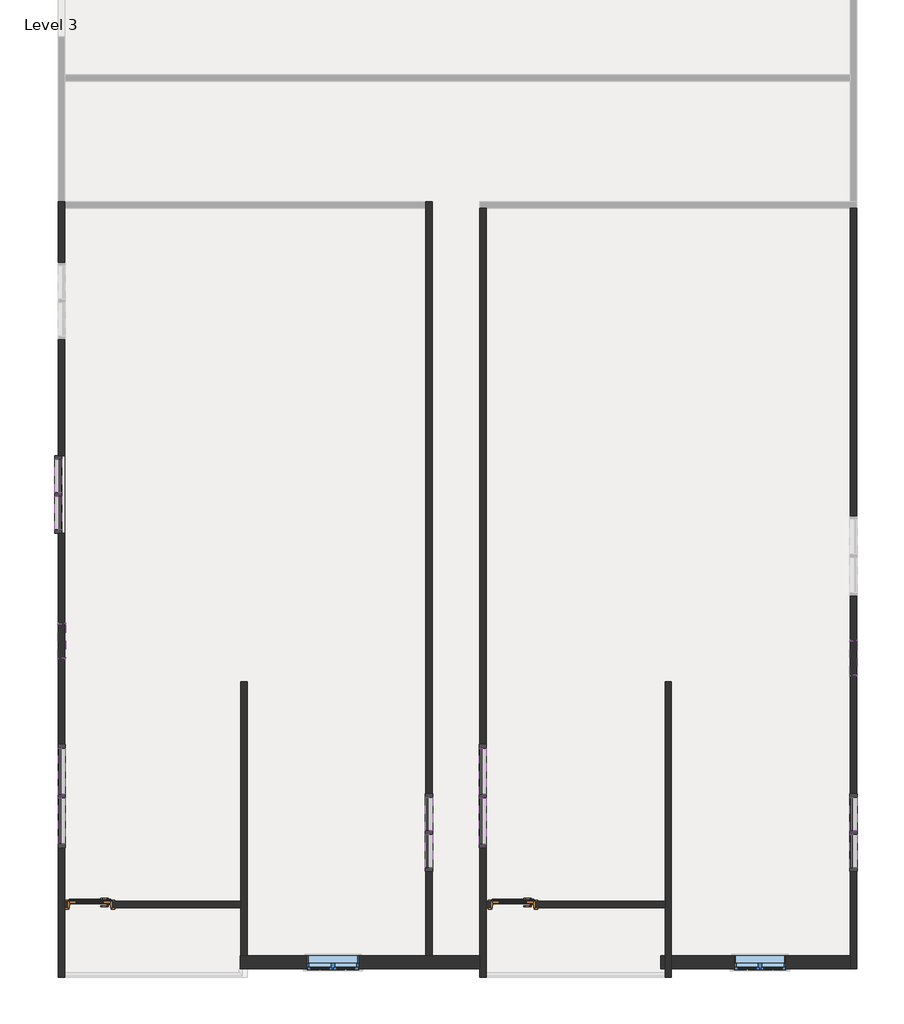
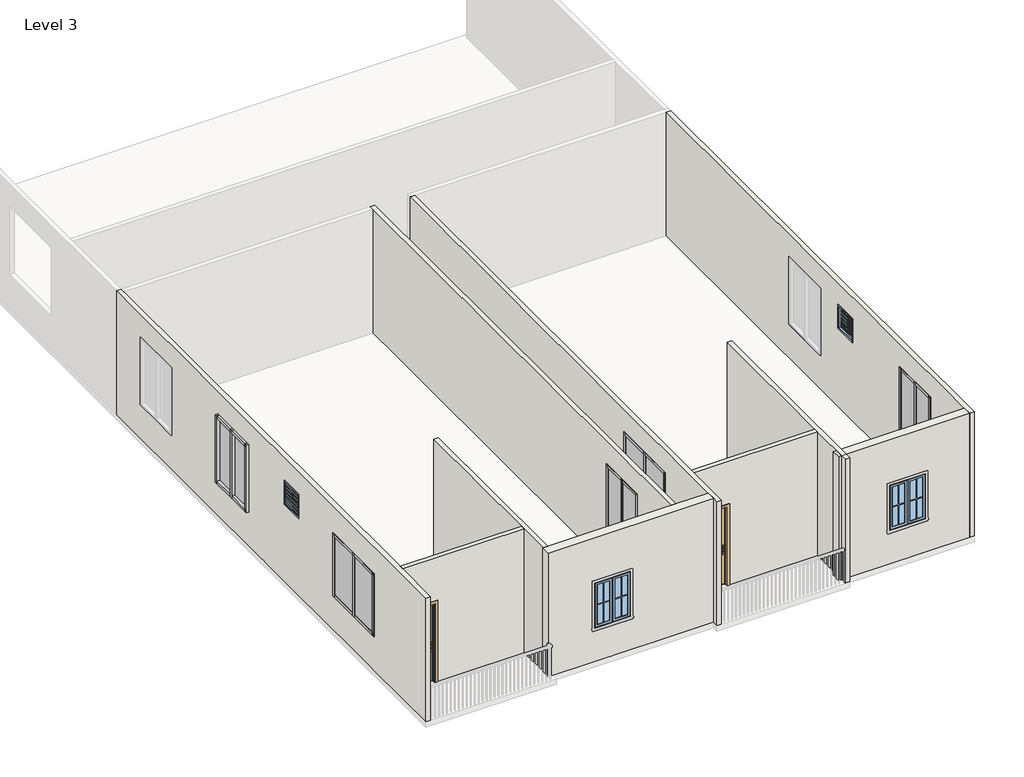
# One storey, part 1 of 3: 35 members, 10 plates, 10 walls, 4 windows, 2 doors.
"""IFC4 building model written with IfcOpenShell, lengths in millimetres."""

from ifc_helpers import new_model, si_unit, frame, origin, place, context, project, spatial, polyline, outline, extrude, faceted_brep, transform, mapped, element, save
from components import door_b81be692, member_8acf8d94, member_501b078b, member_2e6d4a6b, member_96ae0c19, member_d60e8053, member_2fae0574, member_b8ac15de, member_17644e48, system_panel_glazed_c4393626, system_panel_glazed_0e71bc1b, system_panel_glazed_e97abd02, system_panel_glazed_a7ecbca6, window_d341e8ac, window_d39e7ecb

model = new_model("IFC4")

# Units and contexts
model_context = context("Model", 3, world=origin())
ifc_project = project(units=[si_unit("LENGTHUNIT", "METRE", prefix="MILLI")], contexts=[model_context])

# Site, building, storey
site = spatial("IfcSite", under=ifc_project)
building = spatial("IfcBuilding", under=site)
storey = spatial("IfcBuildingStorey", under=building, Name="Level 3", Elevation=6705.6)

# Doors
placement = place(None, origin())
door_shape = door_b81be692(model_context)
element("IfcDoor", 1, ObjectType="29\" x 84\"", at=placement, inside=storey, context=model_context, shape_type="MappedRepresentation", body=[
    mapped(door_shape, transform((-7651.507583, -9448.7163489, 6705.6), x_axis=(1.0, 0.0, 0.0), y_axis=(0.0, 1.0, 0.0), z_axis=(0.0, 0.0, 1.0))),
])
element("IfcDoor", 2, ObjectType="29\" x 84\"", at=placement, inside=storey, context=model_context, shape_type="MappedRepresentation", body=[
    mapped(door_shape, transform((-172.2931282, -9448.9038009, 6705.6), x_axis=(1.0, 0.0, 0.0), y_axis=(0.0, 1.0, 0.0), z_axis=(0.0, 0.0, 1.0))),
])

# Members
member_shape = member_8acf8d94(model_context)
element("IfcMember", 3, ObjectType="Rectangular Mullion : 2.5\" x 5\" rectangular", at=placement, inside=storey, context=model_context, shape_type="MappedRepresentation", body=[
    mapped(member_shape, transform((-8153.157583, -8377.1401329, 9327.486558), x_axis=(0.0, 0.0, 1.0), y_axis=(-1.0, 0.0, 0.0), z_axis=(0.0, -1.0, 0.0))),
])
element("IfcMember", 4, ObjectType="Rectangular Mullion : 2.5\" x 5\" rectangular", at=placement, inside=storey, context=model_context, shape_type="MappedRepresentation", body=[
    mapped(member_shape, transform((-8153.157583, -7497.6651329, 9327.486558), x_axis=(0.0, 0.0, 1.0), y_axis=(-1.0, 0.0, 0.0), z_axis=(0.0, -1.0, 0.0))),
])
element("IfcMember", 5, ObjectType="Rectangular Mullion : 2.5\" x 5\" rectangular", at=placement, inside=storey, context=model_context, shape_type="MappedRepresentation", body=[
    mapped(member_shape, transform((-8153.157583, -6681.6901329, 7620.0), x_axis=(0.0, 0.0, -1.0), y_axis=(-1.0, 0.0, 0.0), z_axis=(0.0, 1.0, 0.0))),
])
element("IfcMember", 6, ObjectType="Rectangular Mullion : 2.5\" x 5\" rectangular", at=placement, inside=storey, context=model_context, shape_type="MappedRepresentation", body=[
    mapped(member_shape, transform((-8153.157583, -7561.1651329, 7620.0), x_axis=(0.0, 0.0, -1.0), y_axis=(-1.0, 0.0, 0.0), z_axis=(0.0, 1.0, 0.0))),
])
member_2_shape = member_501b078b(model_context)
element("IfcMember", 7, ObjectType="Rectangular Mullion : 2.5\" x 5\" rectangular", at=placement, inside=storey, context=model_context, shape_type="MappedRepresentation", body=[
    mapped(member_2_shape, transform((5848.1708786, -8795.0998253, 9448.8), x_axis=(0.0, 0.0, 1.0), y_axis=(-1.0, 0.0, 0.0), z_axis=(0.0, -1.0, 0.0))),
])
element("IfcMember", 8, ObjectType="Rectangular Mullion : 2.5\" x 5\" rectangular", at=placement, inside=storey, context=model_context, shape_type="MappedRepresentation", body=[
    mapped(member_2_shape, transform((5848.1708786, -8142.1745373, 9448.8), x_axis=(0.0, 0.0, 1.0), y_axis=(-1.0, 0.0, 0.0), z_axis=(0.0, -1.0, 0.0))),
])
element("IfcMember", 9, ObjectType="Rectangular Mullion : 2.5\" x 5\" rectangular", at=placement, inside=storey, context=model_context, shape_type="MappedRepresentation", body=[
    mapped(member_2_shape, transform((-1656.4435762, -8795.0998253, 9448.8), x_axis=(0.0, 0.0, 1.0), y_axis=(-1.0, 0.0, 0.0), z_axis=(0.0, -1.0, 0.0))),
])
element("IfcMember", 10, ObjectType="Rectangular Mullion : 2.5\" x 5\" rectangular", at=placement, inside=storey, context=model_context, shape_type="MappedRepresentation", body=[
    mapped(member_2_shape, transform((-1656.4435762, -8142.1745373, 9448.8), x_axis=(0.0, 0.0, 1.0), y_axis=(-1.0, 0.0, 0.0), z_axis=(0.0, -1.0, 0.0))),
])
element("IfcMember", 11, ObjectType="Rectangular Mullion : 2.5\" x 5\" rectangular", at=placement, inside=storey, context=model_context, shape_type="MappedRepresentation", body=[
    mapped(member_2_shape, transform((5848.1708786, -7552.7492493, 7620.0), x_axis=(0.0, 0.0, -1.0), y_axis=(-1.0, 0.0, 0.0), z_axis=(0.0, 1.0, 0.0))),
])
element("IfcMember", 12, ObjectType="Rectangular Mullion : 2.5\" x 5\" rectangular", at=placement, inside=storey, context=model_context, shape_type="MappedRepresentation", body=[
    mapped(member_2_shape, transform((5848.1708786, -8205.6745373, 7620.0), x_axis=(0.0, 0.0, -1.0), y_axis=(-1.0, 0.0, 0.0), z_axis=(0.0, 1.0, 0.0))),
])
element("IfcMember", 13, ObjectType="Rectangular Mullion : 2.5\" x 5\" rectangular", at=placement, inside=storey, context=model_context, shape_type="MappedRepresentation", body=[
    mapped(member_2_shape, transform((-1656.4435762, -7552.7492493, 7620.0), x_axis=(0.0, 0.0, -1.0), y_axis=(-1.0, 0.0, 0.0), z_axis=(0.0, 1.0, 0.0))),
])
element("IfcMember", 14, ObjectType="Rectangular Mullion : 2.5\" x 5\" rectangular", at=placement, inside=storey, context=model_context, shape_type="MappedRepresentation", body=[
    mapped(member_2_shape, transform((-1656.4435762, -8205.6745373, 7620.0), x_axis=(0.0, 0.0, -1.0), y_axis=(-1.0, 0.0, 0.0), z_axis=(0.0, 1.0, 0.0))),
])
member_3_shape = member_2e6d4a6b(model_context)
element("IfcMember", 15, ObjectType="Rectangular Mullion : 2.5\" x 5\" rectangular", at=placement, inside=storey, context=model_context, shape_type="MappedRepresentation", body=[
    mapped(member_3_shape, transform((-705.6931282, -8380.4909009, 9448.8), x_axis=(0.0, 0.0, 1.0), y_axis=(-1.0, 0.0, 0.0), z_axis=(0.0, -1.0, 0.0))),
])
element("IfcMember", 16, ObjectType="Rectangular Mullion : 2.5\" x 5\" rectangular", at=placement, inside=storey, context=model_context, shape_type="MappedRepresentation", body=[
    mapped(member_3_shape, transform((-705.6931282, -7499.3405169, 9448.8), x_axis=(0.0, 0.0, 1.0), y_axis=(-1.0, 0.0, 0.0), z_axis=(0.0, -1.0, 0.0))),
])
element("IfcMember", 17, ObjectType="Rectangular Mullion : 2.5\" x 5\" rectangular", at=placement, inside=storey, context=model_context, shape_type="MappedRepresentation", body=[
    mapped(member_3_shape, transform((-705.6931282, -6681.6901329, 7620.0), x_axis=(0.0, 0.0, -1.0), y_axis=(-1.0, 0.0, 0.0), z_axis=(0.0, 1.0, 0.0))),
])
element("IfcMember", 18, ObjectType="Rectangular Mullion : 2.5\" x 5\" rectangular", at=placement, inside=storey, context=model_context, shape_type="MappedRepresentation", body=[
    mapped(member_3_shape, transform((-705.6931282, -7562.8405169, 7620.0), x_axis=(0.0, 0.0, -1.0), y_axis=(-1.0, 0.0, 0.0), z_axis=(0.0, 1.0, 0.0))),
])
member_4_shape = member_96ae0c19(model_context)
element("IfcMember", 19, ObjectType="Rectangular Mullion : 2.5\" x 5\" rectangular", at=placement, inside=storey, context=model_context, shape_type="MappedRepresentation", body=[
    mapped(member_4_shape, transform((-8210.307583, -2819.4060617, 9448.8), x_axis=(0.0, 0.0, 1.0), y_axis=(-1.0, 0.0, 0.0), z_axis=(0.0, -1.0, 0.0))),
])
element("IfcMember", 20, ObjectType="Rectangular Mullion : 2.5\" x 5\" rectangular", at=placement, inside=storey, context=model_context, shape_type="MappedRepresentation", body=[
    mapped(member_4_shape, transform((-8210.307583, -2164.5788979, 9448.8), x_axis=(0.0, 0.0, 1.0), y_axis=(-1.0, 0.0, 0.0), z_axis=(0.0, -1.0, 0.0))),
])
element("IfcMember", 21, ObjectType="Rectangular Mullion : 2.5\" x 5\" rectangular", at=placement, inside=storey, context=model_context, shape_type="MappedRepresentation", body=[
    mapped(member_4_shape, transform((-8210.307583, -1573.2517341, 7620.0), x_axis=(0.0, 0.0, -1.0), y_axis=(-1.0, 0.0, 0.0), z_axis=(0.0, 1.0, 0.0))),
])
element("IfcMember", 22, ObjectType="Rectangular Mullion : 2.5\" x 5\" rectangular", at=placement, inside=storey, context=model_context, shape_type="MappedRepresentation", body=[
    mapped(member_4_shape, transform((-8210.307583, -2228.0788979, 7620.0), x_axis=(0.0, 0.0, -1.0), y_axis=(-1.0, 0.0, 0.0), z_axis=(0.0, 1.0, 0.0))),
])
member_5_shape = member_d60e8053(model_context)
element("IfcMember", 23, ObjectType="Rectangular Mullion : 2.5\" x 5\" rectangular", at=placement, inside=storey, context=model_context, shape_type="MappedRepresentation", body=[
    mapped(member_5_shape, transform((-8210.307583, -2196.3288979, 7620.0), x_axis=(0.0, -1.0, 0.0), y_axis=(-1.0, 0.0, 0.0), z_axis=(0.0, 0.0, -1.0))),
])
member_6_shape = member_2fae0574(model_context)
element("IfcMember", 24, ObjectType="Rectangular Mullion : 2.5\" x 5\" rectangular", at=placement, inside=storey, context=model_context, shape_type="MappedRepresentation", body=[
    mapped(member_6_shape, transform((-8210.307583, -1509.7517341, 9448.8), x_axis=(0.0, 1.0, 0.0), y_axis=(-1.0, 0.0, 0.0), z_axis=(0.0, 0.0, 1.0))),
])
element("IfcMember", 25, ObjectType="Rectangular Mullion : 2.5\" x 5\" rectangular", at=placement, inside=storey, context=model_context, shape_type="MappedRepresentation", body=[
    mapped(member_6_shape, transform((-8210.307583, -2882.9060617, 7620.0), x_axis=(0.0, -1.0, 0.0), y_axis=(-1.0, 0.0, 0.0), z_axis=(0.0, 0.0, -1.0))),
])
member_7_shape = member_b8ac15de(model_context)
element("IfcMember", 26, ObjectType="Rectangular Mullion : 2.5\" x 5\" rectangular", at=placement, inside=storey, context=model_context, shape_type="MappedRepresentation", body=[
    mapped(member_7_shape, transform((-8153.157583, -7529.4151329, 7620.0), x_axis=(0.0, -1.0, 0.0), y_axis=(-1.0, 0.0, 0.0), z_axis=(0.0, 0.0, -1.0))),
])
member_8_shape = member_17644e48(model_context)
element("IfcMember", 27, ObjectType="Rectangular Mullion : 2.5\" x 5\" rectangular", at=placement, inside=storey, context=model_context, shape_type="MappedRepresentation", body=[
    mapped(member_8_shape, transform((-8153.157583, -6618.1901329, 9327.486558), x_axis=(0.0, 1.0, 0.0), y_axis=(-1.0, 0.0, 0.0), z_axis=(0.0, 0.0, 1.0))),
])
element("IfcMember", 28, ObjectType="Rectangular Mullion : 2.5\" x 5\" rectangular", at=placement, inside=storey, context=model_context, shape_type="MappedRepresentation", body=[
    mapped(member_8_shape, transform((-8153.157583, -8440.6401329, 7620.0), x_axis=(0.0, -1.0, 0.0), y_axis=(-1.0, 0.0, 0.0), z_axis=(0.0, 0.0, -1.0))),
])
element("IfcMember", 29, ObjectType="Rectangular Mullion : 2.5\" x 5\" rectangular", at=placement, inside=storey, context=model_context, shape_type="MappedRepresentation", body=[
    mapped(member_5_shape, transform((5848.1708786, -8173.9245373, 7620.0), x_axis=(0.0, -1.0, 0.0), y_axis=(-1.0, 0.0, 0.0), z_axis=(0.0, 0.0, -1.0))),
])
element("IfcMember", 30, ObjectType="Rectangular Mullion : 2.5\" x 5\" rectangular", at=placement, inside=storey, context=model_context, shape_type="MappedRepresentation", body=[
    mapped(member_5_shape, transform((-1656.4435762, -8173.9245373, 7620.0), x_axis=(0.0, -1.0, 0.0), y_axis=(-1.0, 0.0, 0.0), z_axis=(0.0, 0.0, -1.0))),
])
element("IfcMember", 31, ObjectType="Rectangular Mullion : 2.5\" x 5\" rectangular", at=placement, inside=storey, context=model_context, shape_type="MappedRepresentation", body=[
    mapped(member_5_shape, transform((-705.6931282, -7531.0905169, 7620.0), x_axis=(0.0, -1.0, 0.0), y_axis=(-1.0, 0.0, 0.0), z_axis=(0.0, 0.0, -1.0))),
])
element("IfcMember", 32, ObjectType="Rectangular Mullion : 2.5\" x 5\" rectangular", at=placement, inside=storey, context=model_context, shape_type="MappedRepresentation", body=[
    mapped(member_6_shape, transform((5848.1708786, -7489.2492493, 9448.8), x_axis=(0.0, 1.0, 0.0), y_axis=(-1.0, 0.0, 0.0), z_axis=(0.0, 0.0, 1.0))),
])
element("IfcMember", 33, ObjectType="Rectangular Mullion : 2.5\" x 5\" rectangular", at=placement, inside=storey, context=model_context, shape_type="MappedRepresentation", body=[
    mapped(member_6_shape, transform((-1656.4435762, -7489.2492493, 9448.8), x_axis=(0.0, 1.0, 0.0), y_axis=(-1.0, 0.0, 0.0), z_axis=(0.0, 0.0, 1.0))),
])
element("IfcMember", 34, ObjectType="Rectangular Mullion : 2.5\" x 5\" rectangular", at=placement, inside=storey, context=model_context, shape_type="MappedRepresentation", body=[
    mapped(member_6_shape, transform((-705.6931282, -6618.1901329, 9448.8), x_axis=(0.0, 1.0, 0.0), y_axis=(-1.0, 0.0, 0.0), z_axis=(0.0, 0.0, 1.0))),
])
element("IfcMember", 35, ObjectType="Rectangular Mullion : 2.5\" x 5\" rectangular", at=placement, inside=storey, context=model_context, shape_type="MappedRepresentation", body=[
    mapped(member_6_shape, transform((5848.1708786, -8858.5998253, 7620.0), x_axis=(0.0, -1.0, 0.0), y_axis=(-1.0, 0.0, 0.0), z_axis=(0.0, 0.0, -1.0))),
])
element("IfcMember", 36, ObjectType="Rectangular Mullion : 2.5\" x 5\" rectangular", at=placement, inside=storey, context=model_context, shape_type="MappedRepresentation", body=[
    mapped(member_6_shape, transform((-1656.4435762, -8858.5998253, 7620.0), x_axis=(0.0, -1.0, 0.0), y_axis=(-1.0, 0.0, 0.0), z_axis=(0.0, 0.0, -1.0))),
])
element("IfcMember", 37, ObjectType="Rectangular Mullion : 2.5\" x 5\" rectangular", at=placement, inside=storey, context=model_context, shape_type="MappedRepresentation", body=[
    mapped(member_6_shape, transform((-705.6931282, -8443.9909009, 7620.0), x_axis=(0.0, -1.0, 0.0), y_axis=(-1.0, 0.0, 0.0), z_axis=(0.0, 0.0, -1.0))),
])

# Plates
system_panel_glazed_shape = system_panel_glazed_c4393626(model_context)
element("IfcPlate", 38, ObjectType="System Panel : Glazed", at=placement, inside=storey, context=model_context, shape_type="MappedRepresentation", body=[
    mapped(system_panel_glazed_shape, transform((-8210.307583, -1868.915316, 7683.5), x_axis=(0.0, -1.0, 0.0), y_axis=(1.0, 0.0, 0.0), z_axis=(0.0, 0.0, 1.0))),
])
element("IfcPlate", 39, ObjectType="System Panel : Glazed", at=placement, inside=storey, context=model_context, shape_type="MappedRepresentation", body=[
    mapped(system_panel_glazed_shape, transform((-8210.307583, -2523.7424798, 7683.5), x_axis=(0.0, -1.0, 0.0), y_axis=(1.0, 0.0, 0.0), z_axis=(0.0, 0.0, 1.0))),
])
system_panel_glazed_2_shape = system_panel_glazed_0e71bc1b(model_context)
element("IfcPlate", 40, ObjectType="System Panel : Glazed", at=placement, inside=storey, context=model_context, shape_type="MappedRepresentation", body=[
    mapped(system_panel_glazed_2_shape, transform((-8153.157583, -7089.6776329, 7683.5), x_axis=(0.0, -1.0, 0.0), y_axis=(1.0, 0.0, 0.0), z_axis=(0.0, 0.0, 1.0))),
])
element("IfcPlate", 41, ObjectType="System Panel : Glazed", at=placement, inside=storey, context=model_context, shape_type="MappedRepresentation", body=[
    mapped(system_panel_glazed_2_shape, transform((-8153.157583, -7969.1526329, 7683.5), x_axis=(0.0, -1.0, 0.0), y_axis=(1.0, 0.0, 0.0), z_axis=(0.0, 0.0, 1.0))),
])
system_panel_glazed_3_shape = system_panel_glazed_e97abd02(model_context)
element("IfcPlate", 42, ObjectType="System Panel : Glazed", at=placement, inside=storey, context=model_context, shape_type="MappedRepresentation", body=[
    mapped(system_panel_glazed_3_shape, transform((5848.1708786, -7847.4618933, 7683.5), x_axis=(0.0, -1.0, 0.0), y_axis=(1.0, 0.0, 0.0), z_axis=(0.0, 0.0, 1.0))),
])
element("IfcPlate", 43, ObjectType="System Panel : Glazed", at=placement, inside=storey, context=model_context, shape_type="MappedRepresentation", body=[
    mapped(system_panel_glazed_3_shape, transform((-1656.4435762, -7847.4618933, 7683.5), x_axis=(0.0, -1.0, 0.0), y_axis=(1.0, 0.0, 0.0), z_axis=(0.0, 0.0, 1.0))),
])
element("IfcPlate", 44, ObjectType="System Panel : Glazed", at=placement, inside=storey, context=model_context, shape_type="MappedRepresentation", body=[
    mapped(system_panel_glazed_3_shape, transform((5848.1708786, -8500.3871813, 7683.5), x_axis=(0.0, -1.0, 0.0), y_axis=(1.0, 0.0, 0.0), z_axis=(0.0, 0.0, 1.0))),
])
element("IfcPlate", 45, ObjectType="System Panel : Glazed", at=placement, inside=storey, context=model_context, shape_type="MappedRepresentation", body=[
    mapped(system_panel_glazed_3_shape, transform((-1656.4435762, -8500.3871813, 7683.5), x_axis=(0.0, -1.0, 0.0), y_axis=(1.0, 0.0, 0.0), z_axis=(0.0, 0.0, 1.0))),
])
system_panel_glazed_4_shape = system_panel_glazed_a7ecbca6(model_context)
element("IfcPlate", 46, ObjectType="System Panel : Glazed", at=placement, inside=storey, context=model_context, shape_type="MappedRepresentation", body=[
    mapped(system_panel_glazed_4_shape, transform((-705.6931282, -7090.5153249, 7683.5), x_axis=(0.0, -1.0, 0.0), y_axis=(1.0, 0.0, 0.0), z_axis=(0.0, 0.0, 1.0))),
])
element("IfcPlate", 47, ObjectType="System Panel : Glazed", at=placement, inside=storey, context=model_context, shape_type="MappedRepresentation", body=[
    mapped(system_panel_glazed_4_shape, transform((-705.6931282, -7971.6657089, 7683.5), x_axis=(0.0, -1.0, 0.0), y_axis=(1.0, 0.0, 0.0), z_axis=(0.0, 0.0, 1.0))),
])

# Walls
element("IfcWall", 48, ObjectType="4.5\" wall", at=placement, inside=storey, context=model_context, shape_type="Brep", body=[
    faceted_brep([(-8096.007583, -10738.0280197, 6705.6), (-8096.007583, -9509.0413489, 6705.6), (-8096.007583, -9394.7413489, 6705.6), (-8096.007583, 2864.0002499, 6705.6), (-8096.007583, 2978.3002499, 6705.6), (-8096.007583, 2978.3002499, 10058.4), (-8096.007583, 2864.0002499, 10058.4), (-8096.007583, -9394.7413489, 10058.4), (-8096.007583, -9509.0413489, 10058.4), (-8096.007583, -10738.0280197, 10058.4), (-8096.007583, -6618.1901329, 9327.486558), (-8096.007583, -6618.1901329, 7620.0), (-8096.007583, -8440.6401329, 7620.0), (-8096.007583, -8440.6401329, 9327.486558), (-8096.007583, -5094.1901329, 8820.15), (-8096.007583, -5094.1901329, 9429.75), (-8096.007583, -4484.5901329, 9429.75), (-8096.007583, -4484.5901329, 8820.15), (-8096.007583, 1909.8209543, 9448.8), (-8096.007583, 1909.8209543, 7620.0), (-8096.007583, 536.6666267, 7620.0), (-8096.007583, 536.6666267, 9448.8), (-8096.007583, -1509.7517341, 9448.8), (-8096.007583, -1509.7517341, 7620.0), (-8096.007583, -2882.9060617, 7620.0), (-8096.007583, -2882.9060617, 9448.8), (-8210.307583, 2978.3002499, 6705.6), (-8210.307583, -10738.0280197, 6705.6), (-8210.307583, -10738.0280197, 10058.4), (-8210.307583, 2978.3002499, 10058.4), (-8210.307583, -6618.1901329, 7620.0), (-8210.307583, -6618.1901329, 9327.486558), (-8210.307583, -8440.6401329, 9327.486558), (-8210.307583, -8440.6401329, 7620.0), (-8210.307583, -5094.1901329, 9429.75), (-8210.307583, -5094.1901329, 8820.15), (-8210.307583, -4484.5901329, 8820.15), (-8210.307583, -4484.5901329, 9429.75), (-8210.307583, 1909.8209543, 7620.0), (-8210.307583, 1909.8209543, 9448.8), (-8210.307583, 536.6666267, 9448.8), (-8210.307583, 536.6666267, 7620.0), (-8210.307583, -1509.7517341, 7620.0), (-8210.307583, -1509.7517341, 9448.8), (-8210.307583, -2882.9060617, 9448.8), (-8210.307583, -2882.9060617, 7620.0)], [[[0, 1, 2, 3, 4, 5, 6, 7, 8, 9], [10, 11, 12, 13], [14, 15, 16, 17], [18, 19, 20, 21], [22, 23, 24, 25]], [[26, 27, 28, 29], [30, 31, 32, 33], [34, 35, 36, 37], [38, 39, 40, 41], [42, 43, 44, 45]], [[4, 3, 2, 1, 0, 27, 26]], [[9, 8, 7, 6, 5, 29, 28]], [[0, 9, 28, 27]], [[5, 4, 26, 29]], [[10, 31, 30, 11]], [[31, 10, 13, 32]], [[32, 13, 12, 33]], [[11, 30, 33, 12]], [[35, 34, 15, 14]], [[36, 35, 14, 17]], [[37, 36, 17, 16]], [[34, 37, 16, 15]], [[38, 19, 18, 39]], [[39, 18, 21, 40]], [[40, 21, 20, 41]], [[19, 38, 41, 20]], [[22, 43, 42, 23]], [[43, 22, 25, 44]], [[44, 25, 24, 45]], [[23, 42, 45, 24]]]),
])
element("IfcWall", 49, ObjectType="4.5\" wall", at=placement, inside=storey, context=model_context, shape_type="Brep", body=[
    faceted_brep([(-1599.2935762, -10357.2779557, 6705.6), (-1599.2935762, 2978.3002499, 6705.6), (-1599.2935762, 2978.3002499, 10058.4), (-1599.2935762, -10357.2779557, 10058.4), (-1599.2935762, -7489.2492493, 9448.8), (-1599.2935762, -7489.2492493, 7620.0), (-1599.2935762, -8858.5998253, 7620.0), (-1599.2935762, -8858.5998253, 9448.8), (-1713.5935762, 2978.3002499, 6705.6), (-1713.5935762, 2864.0002499, 6705.6), (-1713.5935762, -10357.2779557, 6705.6), (-1713.5935762, -10357.2779557, 10058.4), (-1713.5935762, 2864.0002499, 10058.4), (-1713.5935762, 2978.3002499, 10058.4), (-1713.5935762, -7489.2492493, 7620.0), (-1713.5935762, -7489.2492493, 9448.8), (-1713.5935762, -8858.5998253, 9448.8), (-1713.5935762, -8858.5998253, 7620.0)], [[[0, 1, 2, 3], [4, 5, 6, 7]], [[8, 9, 10, 11, 12, 13], [14, 15, 16, 17]], [[1, 0, 10, 9, 8]], [[3, 2, 13, 12, 11]], [[2, 1, 8, 13]], [[0, 3, 11, 10]], [[14, 5, 4, 15]], [[15, 4, 7, 16]], [[16, 7, 6, 17]], [[5, 14, 17, 6]]]),
])
element("IfcWall", 50, ObjectType="4.5\" wall", at=placement, inside=storey, context=model_context, shape_type="Brep", body=[
    faceted_brep([(5791.0208786, 2864.0002499, 6705.6), (5791.0208786, -10357.2779557, 6705.6), (5791.0208786, -10585.8779557, 6705.6), (5791.0208786, -10585.8779557, 10058.4), (5791.0208786, -10357.2779557, 10058.4), (5791.0208786, 2864.0002499, 10058.4), (5791.0208786, -7489.2492493, 7620.0), (5791.0208786, -7489.2492493, 9448.8), (5791.0208786, -8858.5998253, 9448.8), (5791.0208786, -8858.5998253, 7620.0), (5791.0208786, -2574.8021821, 7620.0), (5791.0208786, -2574.8021821, 9448.8), (5791.0208786, -3997.2021821, 9448.8), (5791.0208786, -3997.2021821, 7620.0), (5791.0208786, -4784.6021821, 8858.25), (5791.0208786, -4784.6021821, 9467.85), (5791.0208786, -5394.2021821, 9467.85), (5791.0208786, -5394.2021821, 8858.25), (5905.3208786, -10585.8779557, 6705.6), (5905.3208786, 2864.0002499, 6705.6), (5905.3208786, 2864.0002499, 10058.4), (5905.3208786, -10585.8779557, 10058.4), (5905.3208786, -7489.2492493, 9448.8), (5905.3208786, -7489.2492493, 7620.0), (5905.3208786, -8858.5998253, 7620.0), (5905.3208786, -8858.5998253, 9448.8), (5905.3208786, -2574.8021821, 9448.8), (5905.3208786, -2574.8021821, 7620.0), (5905.3208786, -3997.2021821, 7620.0), (5905.3208786, -3997.2021821, 9448.8), (5905.3208786, -4784.6021821, 9467.85), (5905.3208786, -4784.6021821, 8858.25), (5905.3208786, -5394.2021821, 8858.25), (5905.3208786, -5394.2021821, 9467.85)], [[[0, 1, 2, 3, 4, 5], [6, 7, 8, 9], [10, 11, 12, 13], [14, 15, 16, 17]], [[18, 19, 20, 21], [22, 23, 24, 25], [26, 27, 28, 29], [30, 31, 32, 33]], [[2, 1, 0, 19, 18]], [[5, 4, 3, 21, 20]], [[0, 5, 20, 19]], [[3, 2, 18, 21]], [[22, 7, 6, 23]], [[7, 22, 25, 8]], [[8, 25, 24, 9]], [[23, 6, 9, 24]], [[10, 27, 26, 11]], [[11, 26, 29, 12]], [[12, 29, 28, 13]], [[27, 10, 13, 28]], [[31, 30, 15, 14]], [[32, 31, 14, 17]], [[33, 32, 17, 16]], [[30, 33, 16, 15]]]),
])
element("IfcWall", 51, ObjectType="4.5\" wall", at=placement, inside=storey, context=model_context, shape_type="Brep", body=[
    faceted_brep([(-762.8431282, 2864.0002499, 6705.6), (-762.8431282, -10357.2779557, 6705.6), (-762.8431282, -10585.8779557, 6705.6), (-762.8431282, -10737.6531157, 6705.6), (-762.8431282, -10737.6531157, 10058.4), (-762.8431282, -10585.8779557, 10058.4), (-762.8431282, -10357.2779557, 10058.4), (-762.8431282, 2864.0002499, 10058.4), (-762.8431282, -6618.1901329, 7620.0), (-762.8431282, -6618.1901329, 9448.8), (-762.8431282, -8443.9909009, 9448.8), (-762.8431282, -8443.9909009, 7620.0), (-648.5431282, -10737.6531157, 6705.6), (-648.5431282, -9509.2288009, 6705.6), (-648.5431282, -9394.9288009, 6705.6), (-648.5431282, 2864.0002499, 6705.6), (-648.5431282, 2864.0002499, 10058.4), (-648.5431282, -9394.9288009, 10058.4), (-648.5431282, -9509.2288009, 10058.4), (-648.5431282, -10737.6531157, 10058.4), (-648.5431282, -6618.1901329, 9448.8), (-648.5431282, -6618.1901329, 7620.0), (-648.5431282, -8443.9909009, 7620.0), (-648.5431282, -8443.9909009, 9448.8)], [[[0, 1, 2, 3, 4, 5, 6, 7], [8, 9, 10, 11]], [[12, 13, 14, 15, 16, 17, 18, 19], [20, 21, 22, 23]], [[3, 2, 1, 0, 15, 14, 13, 12]], [[4, 3, 12, 19]], [[7, 6, 5, 4, 19, 18, 17, 16]], [[8, 21, 20, 9]], [[9, 20, 23, 10]], [[10, 23, 22, 11]], [[21, 8, 11, 22]], [[0, 7, 16, 15]]]),
])
element("IfcWall", 52, ObjectType="4.5\" wall", at=placement, inside=storey, context=model_context, shape_type="Brep", body=[
    faceted_brep([(-4874.3237038, -10357.2779557, 6705.6), (-4874.3237038, -5507.4946657, 6705.6), (-4874.3237038, -5507.4946657, 10058.4), (-4874.3237038, -10357.2779557, 10058.4), (-4988.6237038, -10357.2779557, 6705.6), (-4988.6237038, -10357.2779557, 10058.4), (-4988.6237038, -9509.0413489, 10058.4), (-4988.6237038, -9394.7413489, 10058.4), (-4988.6237038, -5507.4946657, 10058.4), (-4988.6237038, -5507.4946657, 6705.6), (-4988.6237038, -9394.7413489, 6705.6), (-4988.6237038, -9509.0413489, 6705.6)], [[[0, 1, 2, 3]], [[4, 5, 6, 7, 8, 9, 10, 11]], [[1, 0, 4, 11, 10, 9]], [[2, 1, 9, 8]], [[3, 2, 8, 7, 6, 5]], [[0, 3, 5, 4]]]),
])
element("IfcWall", 53, ObjectType="4.5\" wall", at=placement, inside=storey, context=model_context, shape_type="Brep", body=[
    faceted_brep([(2515.990751, -5507.4946657, 6705.6), (2515.990751, -9394.9288009, 6705.6), (2515.990751, -9509.2288009, 6705.6), (2515.990751, -10737.6531157, 6705.6), (2515.990751, -10737.6531157, 10058.4), (2515.990751, -9509.2288009, 10058.4), (2515.990751, -9394.9288009, 10058.4), (2515.990751, -5507.4946657, 10058.4), (2630.290751, -5507.4946657, 6705.6), (2630.290751, -5507.4946657, 10058.4), (2630.290751, -10737.6531157, 10058.4), (2630.290751, -10737.6531157, 6705.6)], [[[0, 1, 2, 3, 4, 5, 6, 7]], [[8, 9, 10, 11]], [[3, 2, 1, 0, 8, 11]], [[4, 3, 11, 10]], [[7, 6, 5, 4, 10, 9]], [[0, 7, 9, 8]]]),
])
element("IfcWall", 54, ObjectType="4.5\" wall", at=placement, inside=storey, context=model_context, shape_type="SweptSolid", body=[
    extrude(outline(polyline([(10058.4, -4988.6237038), (10058.4, -8096.007583), (6705.6, -8096.007583), (6705.6, -8045.207583), (8864.6, -8045.207583), (8864.6, -7257.807583), (6705.6, -7257.807583), (6705.6, -4988.6237038), (10058.4, -4988.6237038)])), frame((0.0, -9509.0413489, 0.0), z_axis=(0.0, 1.0, 0.0), x_axis=(0.0, 0.0, 1.0)), (0.0, 0.0, 1.0), 114.3),
])
element("IfcWall", 55, ObjectType="4.5\" wall", at=placement, inside=storey, context=model_context, shape_type="SweptSolid", body=[
    extrude(outline(polyline([(10058.4, 2515.990751), (10058.4, -648.5431282), (6705.6, -648.5431282), (6705.6, -565.9931282), (8864.6, -565.9931282), (8864.6, 221.4068718), (6705.6, 221.4068718), (6705.6, 2515.990751), (10058.4, 2515.990751)])), frame((0.0, -9509.2288009, 0.0), z_axis=(0.0, 1.0, 0.0), x_axis=(0.0, 0.0, 1.0)), (0.0, 0.0, 1.0), 114.3),
])
element("IfcWall", 56, ObjectType="9\" wall", at=placement, inside=storey, context=model_context, shape_type="Brep", body=[
    faceted_brep([(-762.8431282, -10357.2779557, 6705.6), (-1599.2935762, -10357.2779557, 6705.6), (-1713.5935762, -10357.2779557, 6705.6), (-4874.3237038, -10357.2779557, 6705.6), (-4988.6237038, -10357.2779557, 6705.6), (-4996.231207, -10357.2779557, 6705.6), (-4996.231207, -10357.2779557, 10058.4), (-4988.6237038, -10357.2779557, 10058.4), (-4874.3237038, -10357.2779557, 10058.4), (-1713.5935762, -10357.2779557, 10058.4), (-1599.2935762, -10357.2779557, 10058.4), (-762.8431282, -10357.2779557, 10058.4), (-3813.8737038, -10357.2779557, 8839.2), (-3813.8737038, -10357.2779557, 7620.0), (-2899.4737038, -10357.2779557, 7620.0), (-2899.4737038, -10357.2779557, 8839.2), (-762.8431282, -10585.8779557, 6705.6), (-762.8431282, -10585.8779557, 10058.4), (-4996.231207, -10585.8779557, 10058.4), (-4996.231207, -10585.8779557, 6705.6), (-3813.8737038, -10585.8779557, 8839.2), (-2899.4737038, -10585.8779557, 8839.2), (-2899.4737038, -10585.8779557, 7620.0), (-3813.8737038, -10585.8779557, 7620.0)], [[[0, 1, 2, 3, 4, 5, 6, 7, 8, 9, 10, 11], [12, 13, 14, 15]], [[16, 17, 18, 19], [20, 21, 22, 23]], [[5, 4, 3, 2, 1, 0, 16, 19]], [[6, 5, 19, 18]], [[11, 10, 9, 8, 7, 6, 18, 17]], [[0, 11, 17, 16]], [[13, 12, 20, 23]], [[14, 13, 23, 22]], [[15, 14, 22, 21]], [[12, 15, 21, 20]]]),
])
element("IfcWall", 57, ObjectType="9\" wall", at=placement, inside=storey, context=model_context, shape_type="SweptSolid", body=[
    extrude(outline(polyline([(6705.6, 5791.0208786), (10058.4, 5791.0208786), (10058.4, 2436.2994194), (6705.6, 2436.2994194), (6705.6, 5791.0208786)]), holes=[polyline([(8839.2, 3739.9708786), (8839.2, 4654.3708786), (7620.0, 4654.3708786), (7620.0, 3739.9708786), (8839.2, 3739.9708786)])]), frame((0.0, -10585.8779557, 0.0), z_axis=(0.0, 1.0, 0.0), x_axis=(0.0, 0.0, 1.0)), (0.0, 0.0, 1.0), 228.6),
])

# Windows
window_shape = window_d341e8ac(model_context)
element("IfcWindow", 58, ObjectType="Window-Casement-Double : 36\" x 48\"", at=placement, inside=storey, context=model_context, shape_type="MappedRepresentation", body=[
    mapped(window_shape, transform((-3356.6737038, -10471.5779557, 6705.6), x_axis=(-1.0, 0.0, 0.0), y_axis=(0.0, -1.0, 0.0), z_axis=(0.0, 0.0, 1.0))),
])
element("IfcWindow", 59, ObjectType="Window-Casement-Double : 36\" x 48\"", at=placement, inside=storey, context=model_context, shape_type="MappedRepresentation", body=[
    mapped(window_shape, transform((4197.1708786, -10471.5779557, 6705.6), x_axis=(-1.0, 0.0, 0.0), y_axis=(0.0, -1.0, 0.0), z_axis=(0.0, 0.0, 1.0))),
])
window_2_shape = window_d39e7ecb(model_context)
element("IfcWindow", 60, ObjectType="Window-Louvers : 24\" x 24\"", at=placement, inside=storey, context=model_context, shape_type="MappedRepresentation", body=[
    mapped(window_2_shape, transform((-8159.507583, -4789.3901329, 7905.75), x_axis=(0.0, 1.0, 0.0), y_axis=(-1.0, 0.0, 0.0), z_axis=(0.0, 0.0, 1.0))),
])
element("IfcWindow", 61, ObjectType="Window-Louvers : 24\" x 24\"", at=placement, inside=storey, context=model_context, shape_type="MappedRepresentation", body=[
    mapped(window_2_shape, transform((5854.5208786, -5089.4021821, 7943.85), x_axis=(0.0, -1.0, 0.0), y_axis=(1.0, 0.0, 0.0), z_axis=(0.0, 0.0, 1.0))),
])

save(model, "model.ifc")

# Revit data of these elements
# Type "29\" x 84\""
#   Type Mark = "8"
#   Assembly Code = "B2030100"
#   Analytic Construction = "French door, wood frame with single glass"
#   Threshold Offset [instance default] = 0' - 0 1/2"
#   Thickness = 0' - 1 3/8"
#   Thermal Resistance (R) = 1.0696 (h·ft²·°F)/BTU
#   Swing Angle [instance default] = 90.00°
#   Stiles = 0' - 4 3/4"
#   Rough Width = 2' - 7"
#   Rough Height = 7' - 1"
#   Radius = 1' - 0.00625"
#   Lock Rail = 0' - 7 1/8"
#   Height = 7' - 0"
#   Width = 2' - 5"
#   Heat Transfer Coefficient (U) = 0.9350 BTU/(h·ft²·°F)
#   Door Offset [instance default] = 0' - 0"
#   Bottom Rail = 0' - 9 1/2"
#   Threshold [instance default] = yes
#   Function = 1
#   Exterior Trim [instance default] = yes
#   Trim Material = Cherry
#   Threshold Material = Cherry
#   Panel Material = Cherry
#   Glazing = Glass
#   Frame Material = Cherry
#   Door Handle Material = Aluminum
#   Visual Light Transmittance = 0
#   Solar Heat Gain Coefficient = 0
#   Wall Closure = (empty or 0)
#   Construction Type = (empty or 0)
# Type "Rectangular Mullion : 2.5\" x 5\" rectangular"
#   built-in parameter 1007304 = 0.416667 (stored number, unit not read)
#   built-in parameter 1007301 = 0.104167 (stored number, unit not read)
#   built-in parameter 1007300 = 0.104167 (stored number, unit not read)
# Type "System Panel : Glazed"
#   Construction Type Id = "GSP4R"
#   Analytic Construction = "1/8 in Pilkington single glazing"
#   Visual Light Transmittance = 0.9
#   Solar Heat Gain Coefficient = 0.86
#   Heat Transfer Coefficient (U) = 1.18115 BTU/(h·ft²·°F)
#   Define Thermal Properties by = 1
# Type "4.5\" wall"
#   Assembly Code = "B2010"
#   Layers, outside or top first: 0' - 4 1/2" no material (function 1)
# Type "9\" wall"
#   Assembly Code = "B2010"
#   Layers, outside or top first: 0' - 9" no material (function 1)
# Type "Window-Casement-Double : 36\" x 48\""
#   Type Mark = "14"
#   Fire Rating = "0.5h"
#   Assembly Code = "B2020100"
#   Analytic Construction = "Double glazing - domestic"
#   Frame Extension [instance default] = 0' - 0 1/4"
#   Window Inset [instance default] = 0' - 0"
#   Wall Thickness [instance default] = 0' - 6"
#   Interior Wall Closure [instance default] = 0' - 2 1/4"
#   Half Width = 1' - 6"
#   Visual Light Transmittance = 0.81
#   Thermal Resistance (R) = 1.8146 (h·ft²·°F)/BTU
#   Solar Heat Gain Coefficient = 0.76
#   Rough Width = 3' - 0 1/2"
#   Rough Height = 4' - 0 1/2"
#   Height = 4' - 0"
#   Heat Transfer Coefficient (U) = 0.5511 BTU/(h·ft²·°F)
#   Exterior Wall Closure [instance default] = 0' - 1 1/4"
#   Extension Jamb [instance default] = 0' - 2 1/4"
#   Default Sill Height = 3' - 0"
#   Width = 3' - 0"
#   Define Thermal Properties by = 0
#   Muntin Visibility = yes
#   Interior Trim Visibility [instance default] = yes
#   Exterior Trim Visibility [instance default] = yes
#   Extension Jamb Visibility [instance default] = yes
#   Interior Trim Material = Wood - Stained
#   Muntin Pattern = Muntin Pattern_2x2 : Muntin Pattern_2x2
#   Interior Trim = Trim-Window-Interior-Flat : Picture Frame
#   Interior Frame Material = Wood - Stained
#   Glass Panel Material = Glass
#   Exterior Trim Material = Clad - White
#   Exterior Trim = Trim-Window-Exterior-Flat : with Sill
#   Exterior Frame Material = Clad - White
#   Wall Closure = (empty or 0)
# Type "Window-Louvers : 24\" x 24\""
#   Type Mark = "18"
#   Construction Type Id = "GSP4R"
#   Assembly Code = "B20"
#   Analytic Construction = "1/8 in Pilkington single glazing"
#   Visual Light Transmittance = 0.9
#   Thermal Resistance (R) = 1.53941 (h·ft²·°F)/BTU
#   Solar Heat Gain Coefficient = 0.78
#   Max Height = 1' - 11.74264"
#   Height = 2' - 0"
#   Heat Transfer Coefficient (U) = 0.6496 BTU/(h·ft²·°F)
#   Blade Width [instance default] = 1' - 10 1/2"
#   Blade Vertical Thickness = 0' - 0.35355"
#   Blade Thickness = 0' - 0 1/4"
#   Blade Spacing = 0' - 1 1/2"
#   Blade Height = 0' - 1.85355"
#   Blade Depth = 0' - 3"
#   Blade Angle = 45.00°
#   Default Sill Height = 3' - 0"
#   Trim Projection_Exterior = 0' - 0 1/2"
#   Trim Projection_Interior = 0' - 0 1/2"
#   Trim Width_Exterior = 0' - 1 1/2"
#   Trim Width_Interior = 0' - 1 1/2"
#   Width = 2' - 0"
#   Max Blade Count = 12
#   Define Thermal Properties by = 1
#   Blade Count = 12
#   Frame Material = Birch
#   Louver Material = Birch
#   Trim Exterior Material = Birch
#   Trim Interior Material = Birch
#   Wall Closure = (empty or 0)
# Elements 1, 2 (IfcDoor, "29\" x 84\"")
#   Threshold Offset = 0' - 0 1/2"
#   Swing Angle = 90.00°
#   Door Offset = 0' - 0"
#   Threshold = yes
#   Exterior Trim = yes
#   Phase Created = New Construction
#   Materials on its faces: "Cherry", "Aluminum", "Glass"
# Elements 3, 4, 5, 6, 7, 8, 9, 10, 11, 12, 13, 14, 15, 16, 17, 18, 19, 20, 21, 22, 23, 24, 25, 26, 27, 28, 29, 30, 31, 32, 33, 34, 35, 36, 37 (IfcMember, "Rectangular Mullion : 2.5\" x 5\" rectangular")
#   Phase Created = New Construction
#   Materials on its faces: "Aluminum"
# Elements 38, 39, 40, 41, 42, 43, 44, 45, 46, 47 (IfcPlate, "System Panel : Glazed")
#   Phase Created = New Construction
#   Materials on its faces: "Glass"
# Elements 48, 49, 50, 51, 52, 53, 54, 55 (IfcWall, "4.5\" wall")
#   Top Offset = 0' - 0"
#   Base Offset = 0' - 0"
#   wall height = 11' - 0"
#   Phase Created = New Construction
#   Base Constraint = Level 3
#   Top Constraint = Level 4
#   Materials on its faces: "Default Wall"
# Elements 56, 57 (IfcWall, "9\" wall")
#   Top Offset = 0' - 0"
#   Base Offset = 0' - 0"
#   wall height = 11' - 0"
#   Phase Created = New Construction
#   Base Constraint = Level 3
#   Top Constraint = Level 4
#   Materials on its faces: "Default Wall"
# Element 58 (IfcWindow, "Window-Casement-Double : 36\" x 48\"")
#   Mark = "9"
#   Window Inset = 0' - 0"
#   Interior Wall Closure = 0' - 2 1/4"
#   Frame Extension = 0' - 0 1/4"
#   Exterior Wall Closure = 0' - 1 1/4"
#   Interior Trim Visibility = yes
#   Exterior Trim Visibility = yes
#   Phase Created = New Construction
#   Materials on its faces: "Wood - Stained", "Glass", "Clad - White"
# Element 59 (IfcWindow, "Window-Casement-Double : 36\" x 48\"")
#   Mark = "10"
#   Window Inset = 0' - 0"
#   Interior Wall Closure = 0' - 2 1/4"
#   Frame Extension = 0' - 0 1/4"
#   Exterior Wall Closure = 0' - 1 1/4"
#   Interior Trim Visibility = yes
#   Exterior Trim Visibility = yes
#   Phase Created = New Construction
#   Materials on its faces: "Wood - Stained", "Glass", "Clad - White"
# Element 60 (IfcWindow, "Window-Louvers : 24\" x 24\"")
#   Mark = "11"
#   Blade Width = 1' - 10 1/2"
#   Phase Created = New Construction
#   Materials on its faces: "Birch"
# Element 61 (IfcWindow, "Window-Louvers : 24\" x 24\"")
#   Mark = "12"
#   Blade Width = 1' - 10 1/2"
#   Phase Created = New Construction
#   Materials on its faces: "Birch"
# Materials
#   "Cherry": class "Wood", colour RGB 226 177 128, transparency 0, Description = "Prunus Serotina", Cost = 0
#   "Glass": class "Glass", colour RGB 0 128 192, transparency 0.75, Description = "Soda Lime Glass", Cost = 0
#   "Aluminum": class "Metal", colour RGB 247 247 247, transparency 0, Description = "Aluminum 6061", Cost = 0
#   "Wood - Stained": class "Wood", colour RGB 224 178 126, transparency 0, Cost = 0
#   "Clad - White": class "Wood", colour RGB 242 242 238, transparency 0, Cost = 0
#   "Birch": class "Wood", colour RGB 224 178 126, transparency 0, Description = "Betula Alleghaniensis", Cost = 0
#   "Default Wall": colour RGB 128 128 128, transparency 0, Cost = 0
